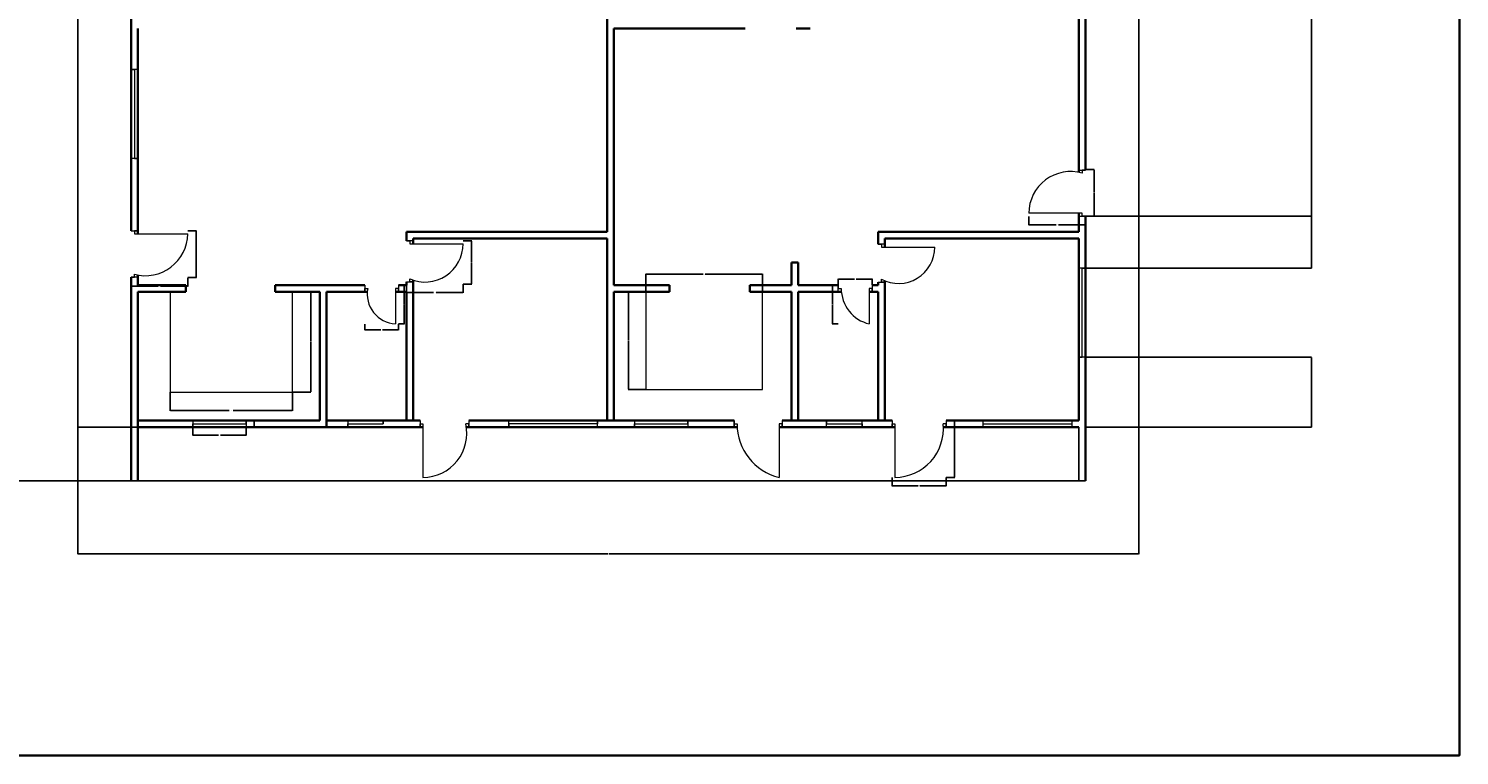
# Model space of a CAD drawing. Units: inches. Extents: x 1520 to 3401, y 1570 to 3432.
# Tile 10 of 15: x 2435 to 3401, y 1570 to 2061. Entities that reach past the tile are written whole.
import ezdxf

# ---------------------------------------------------------------- set-up
doc = ezdxf.new("R2010")
doc.units = ezdxf.units.IN
for name, color, linetype, lineweight in [('A-ANNO-DIMS', 2, 'Continuous', 18), ('A-ANNO-TTLB', 7, 'Continuous', 35), ('A-DOOR', 3, 'Continuous', 18), ('A-FLOR-CASE', 8, 'Continuous', 18), ('A-FLOR-EDGE', 7, 'Continuous', 25), ('A-GLAZ', 4, 'Continuous', 18), ('A-WALL', 7, 'Continuous', 35)]:
    doc.layers.add(name, color=color, linetype=linetype, lineweight=lineweight)
doc.styles.get("Standard").update_dxf_attribs({"font": 'arial.ttf'})
doc.dimstyles.get("Standard").update_dxf_attribs({"dimtxt": 0.18, "dimasz": 0.18, "dimexe": 0.18, "dimexo": 0.0625, "dimgap": 0.09, "dimtad": 0, "dimtih": 1, "dimtoh": 1, "dimdec": 4, "dimzin": 0, "dimdsep": 46, "dimtxsty": 'Standard', "dimcen": 0.09, "dimadec": 0, "dimazin": 0, "dimtfac": 1, "dimtdec": 4, "dimtofl": 0, "dimtmove": 0, "dimatfit": 3, "dimfxl": 1, "dimtolj": 1, "dimtzin": 0, "dimarcsym": 0})

# ---------------------------------------------------------------- blocks, each defined once
blk = doc.blocks.new('DOOR-SWING-24-10')
for p, q in [((0, 21.75), (0, 26.25)), ((0, 26.25), (0, 24)), ((0, 24), (2, 24)), ((23.01, 24), (21.01, 24)), ((21.01, 24), (21.01, 0)), ((23.01, 26.25), (23.01, 21.75)), ((23.01, 21.75), (23.01, 24))]:
    blk.add_line(p, q)
blk.add_arc((26.65, 24), 24.65, 180, 256.77726)
blk = doc.blocks.new('DOOR-SWING-36-11')
for p, q in [((4.5, 26.53), (0, 26.53)), ((0, 26.53), (2.25, 26.53)), ((2.25, 26.53), (2.25, 24.53)), ((2.25, 24.53), (38.25, 24.53)), ((0, 0.83), (4.5, 0.83)), ((2.25, 0.83), (2.25, 2.83)), ((4.5, 0.83), (2.25, 0.83))]:
    blk.add_line(p, q)
blk.add_arc((13.71, 24.53), 24.54, 242.16732, 0)
blk = doc.blocks.new('DOOR-SWING-24-12')
for p, q in [((0, 26.25), (0, 21.75)), ((0, 21.75), (0, 24)), ((0, 24), (2, 24)), ((22.75, 24), (20.75, 24)), ((20.75, 24), (20.75, 0)), ((22.75, 26.25), (22.75, 21.75)), ((22.75, 21.75), (22.75, 24))]:
    blk.add_line(p, q)
blk.add_arc((21.91, 20.23), 20.26, 169.27026, 266.73788)
blk = doc.blocks.new('DOOR-SWING-36-13')
for p, q in [((4.5, 27.75), (0, 27.75)), ((0, 27.75), (2.25, 27.75)), ((2.25, 27.75), (2.25, 25.75)), ((2.25, 25.75), (38.25, 25.75)), ((0, 0.11), (4.5, 0.11)), ((2.25, 0.11), (2.25, 2.11)), ((4.5, 0.11), (2.25, 0.11))]:
    blk.add_line(p, q)
blk.add_arc((12.49, 25.75), 25.76, 246.58617, 0)
blk = doc.blocks.new('DOOR-SWING-36-26')
for p, q in [((0, 31.26), (4.5, 31.26)), ((4.5, 31.26), (2.25, 31.26)), ((2.25, 31.26), (2.25, 29.26)), ((2.25, 29.26), (38.25, 29.26)), ((2.25, 0), (2.25, 2)), ((4.5, 0), (0, 0)), ((0, 0), (2.25, 0))]:
    blk.add_line(p, q)
blk.add_arc((9.61, 29.68), 28.64, 255.11352, 359.16031)
blk = doc.blocks.new('DOOR-SWING-36-27')
for p, q in [((0, 38.25), (0, 33.75)), ((0, 33.75), (0, 36)), ((0, 36), (2, 36)), ((2, 36), (2, 0)), ((36.5, 36), (34.5, 36)), ((36.5, 38.25), (36.5, 33.75)), ((36.5, 33.75), (36.5, 36))]:
    blk.add_line(p, q)
blk.add_arc((2, 32.67), 32.67, 270, 5.84902)
blk = doc.blocks.new('DOOR-SWING-36-28')
for p, q in [((0, 33.75), (0, 38.25)), ((0, 38.25), (0, 33.75)), ((0, 33.75), (0, 36)), ((0, 36), (2, 36)), ((32.37, 36), (30.37, 36)), ((30.37, 36), (30.37, 0)), ((32.37, 38.25), (32.37, 33.75)), ((32.37, 33.75), (32.37, 36))]:
    blk.add_line(p, q)
blk.add_arc((39.03, 36), 37.03, 180, 256.47101)
blk = doc.blocks.new('DOOR-SWING-36-29')
for p, q in [((0, 38.25), (0, 34.72)), ((0, 33.75), (0, 36)), ((0, 36), (2, 36)), ((0, 34.72), (0, 33.75)), ((2, 36), (2, 0)), ((32.89, 36), (30.89, 36)), ((32.89, 38.25), (32.89, 33.75)), ((32.89, 33.75), (32.89, 36))]:
    blk.add_line(p, q)
blk.add_arc((2, 29.59), 29.59, 270, 12.50405)
blk = doc.blocks.new('DOOR-SWING-36-30')
for p, q in [((33.75, 31.05), (38.25, 31.05)), ((38.25, 31.05), (36, 31.05)), ((36, 31.05), (36, 29.05)), ((36, 2), (0, 2)), ((33.75, 0), (38.25, 0)), ((36, 0), (36, 2)), ((38.25, 0), (36, 0))]:
    blk.add_line(p, q)
blk.add_arc((28.16, 2), 28.16, 73.84326, 180)
blk = doc.blocks.new('WIN-PLAN-24-01')
for p, q in [((0, 4.5), (0, 0)), ((0, 0), (0, 2.25)), ((0, 2.25), (24, 2.25)), ((24, 2.25), (24, 4.5)), ((24, 4.5), (24, 0))]:
    blk.add_line(p, q)
blk = doc.blocks.new('WIN-PLAN-60-02')
for p, q in [((4.5, 60), (0, 60)), ((0, 60), (2.25, 60)), ((2.25, 60), (2.25, 0)), ((4.5, 0), (0, 0)), ((2.25, 0), (4.5, 0))]:
    blk.add_line(p, q)
blk = doc.blocks.new('WIN-PLAN-36-04')
for p, q in [((0, 4.5), (0, 0)), ((0, 0), (0, 2.25)), ((0, 2.25), (36, 2.25)), ((36, 2.25), (36, 4.5)), ((36, 4.5), (36, 0))]:
    blk.add_line(p, q)
blk = doc.blocks.new('WIN-PLAN-60-05')
for p, q in [((0, 4.5), (0, 0)), ((0, 2.25), (60, 2.25)), ((60, 4.5), (60, 0))]:
    blk.add_line(p, q)
blk = doc.blocks.new('WIN-PLAN-24-06')
for p, q in [((0, 4.5), (0, 0)), ((0, 0), (0, 2.25)), ((0, 2.25), (24, 2.25)), ((24, 2.25), (24, 4.5)), ((24, 4.5), (24, 2.25))]:
    blk.add_line(p, q)
blk = doc.blocks.new('KITCHEN-COUNTER-01')
for p, q in [((0, 67.75), (0, 0)), ((82.51, 0), (82.51, 67.75)), ((0, 0), (82.51, 0))]:
    blk.add_line(p, q)
blk = doc.blocks.new('KITCHEN-COUNTER-02')
for p, q in [((0, 65.95), (0, 0)), ((78.77, 0), (78.77, 65.95)), ((0, 0), (78.77, 0))]:
    blk.add_line(p, q)
blk = doc.blocks.new('*D71')
at = {"layer": 'A-ANNO-DIMS', "color": 0, "lineweight": -2, "transparency": 16777216}
for p, q in [((2545.58, 1791.62), (2545.58, 1786.1)), ((2581.58, 1791.62), (2581.58, 1786.1)), ((2545.76, 1786.28), (2562.83, 1786.28)), ((2581.4, 1786.28), (2564.34, 1786.28))]:
    blk.add_line(p, q, dxfattribs=at)
at = {"layer": 'A-ANNO-DIMS', "color": 0, "transparency": 16777216}
for points in [[(2545.76, 1786.31), (2545.76, 1786.25), (2545.58, 1786.28)], [(2581.4, 1786.31), (2581.4, 1786.25), (2581.58, 1786.28)]]:
    blk.add_solid(points, dxfattribs=at)
at = {"layer": 'Defpoints', "color": 0, "transparency": 16777216}
for p in [(2545.58, 1791.68), (2581.58, 1791.68), (2581.58, 1786.28)]:
    blk.add_point(p, dxfattribs=at)
at = {"layer": 'A-ANNO-DIMS', "color": 0, "transparency": 16777216, "insert": (2563.58, 1786.28), "char_height": 0.18, "attachment_point": 5}
blk.add_mtext('\\A1;W4 36 TYP.', dxfattribs=at)
blk = doc.blocks.new('*D72')
at = {"layer": 'A-ANNO-DIMS', "color": 0, "lineweight": -2, "transparency": 16777216}
for p, q in [((2581.64, 1796.18), (2587.16, 1796.18)), ((2581.64, 1791.68), (2587.16, 1791.68)), ((2586.98, 1796), (2586.98, 1794.11)), ((2586.98, 1791.86), (2586.98, 1793.75))]:
    blk.add_line(p, q, dxfattribs=at)
at = {"layer": 'A-ANNO-DIMS', "color": 0, "transparency": 16777216}
for points in [[(2586.95, 1796), (2587.01, 1796), (2586.98, 1796.18)], [(2586.95, 1791.86), (2587.01, 1791.86), (2586.98, 1791.68)]]:
    blk.add_solid(points, dxfattribs=at)
at = {"layer": 'Defpoints', "color": 0, "transparency": 16777216}
for p in [(2581.58, 1796.18), (2581.58, 1791.68), (2586.98, 1796.18)]:
    blk.add_point(p, dxfattribs=at)
at = {"layer": 'A-ANNO-DIMS', "color": 0, "transparency": 16777216, "insert": (2586.98, 1793.93), "char_height": 0.18, "attachment_point": 5}
blk.add_mtext('\\A1;5 TYP.', dxfattribs=at)
blk = doc.blocks.new('*D99')
at = {"layer": 'A-ANNO-DIMS', "color": 0, "lineweight": -2, "transparency": 16777216}
for p, q in [((2981.34, 1887.68), (2977.28, 1887.68)), ((2977.46, 1887.5), (2977.46, 1874.74)), ((2977.46, 1861.61), (2977.46, 1874.37)), ((2981.34, 1861.43), (2977.28, 1861.43))]:
    blk.add_line(p, q, dxfattribs=at)
at = {"layer": 'A-ANNO-DIMS', "color": 0, "transparency": 16777216}
for points in [[(2977.43, 1887.5), (2977.49, 1887.5), (2977.46, 1887.68)], [(2977.43, 1861.61), (2977.49, 1861.61), (2977.46, 1861.43)]]:
    blk.add_solid(points, dxfattribs=at)
at = {"layer": 'Defpoints', "color": 0, "transparency": 16777216}
for p in [(2977.46, 1887.68), (2981.4, 1887.68), (2981.4, 1861.43)]:
    blk.add_point(p, dxfattribs=at)
at = {"layer": 'A-ANNO-DIMS', "color": 0, "transparency": 16777216, "insert": (2977.46, 1874.55), "char_height": 0.18, "attachment_point": 5}
blk.add_mtext('\\A1;D10 26 TYP.', dxfattribs=at)
blk = doc.blocks.new('*D100')
at = {"layer": 'A-ANNO-DIMS', "color": 0, "lineweight": -2, "transparency": 16777216}
for p, q in [((2981.4, 1887.74), (2981.4, 1891.8)), ((2981.58, 1891.62), (2992.38, 1891.62)), ((3004.23, 1891.62), (2993.44, 1891.62)), ((3004.41, 1887.74), (3004.41, 1891.8))]:
    blk.add_line(p, q, dxfattribs=at)
at = {"layer": 'A-ANNO-DIMS', "color": 0, "transparency": 16777216}
for points in [[(2981.58, 1891.65), (2981.58, 1891.59), (2981.4, 1891.62)], [(3004.23, 1891.65), (3004.23, 1891.59), (3004.41, 1891.62)]]:
    blk.add_solid(points, dxfattribs=at)
at = {"layer": 'Defpoints', "color": 0, "transparency": 16777216}
for p in [(2981.4, 1887.68), (3004.41, 1891.62), (3004.41, 1887.68)]:
    blk.add_point(p, dxfattribs=at)
at = {"layer": 'A-ANNO-DIMS', "color": 0, "transparency": 16777216, "insert": (2992.91, 1891.62), "char_height": 0.18, "attachment_point": 5}
blk.add_mtext('\\A1;23 TYP.', dxfattribs=at)
blk = doc.blocks.new('*D103')
at = {"layer": 'A-ANNO-DIMS', "color": 0, "lineweight": -2, "transparency": 16777216}
for p, q in [((2684.52, 1887.68), (2688.57, 1887.68)), ((2688.39, 1887.5), (2688.39, 1874.74)), ((2688.39, 1861.61), (2688.39, 1874.37)), ((2684.52, 1861.43), (2688.57, 1861.43))]:
    blk.add_line(p, q, dxfattribs=at)
at = {"layer": 'A-ANNO-DIMS', "color": 0, "transparency": 16777216}
for points in [[(2688.36, 1887.5), (2688.42, 1887.5), (2688.39, 1887.68)], [(2688.36, 1861.61), (2688.42, 1861.61), (2688.39, 1861.43)]]:
    blk.add_solid(points, dxfattribs=at)
at = {"layer": 'Defpoints', "color": 0, "transparency": 16777216}
for p in [(2684.45, 1887.68), (2688.39, 1887.68), (2684.45, 1861.43)]:
    blk.add_point(p, dxfattribs=at)
at = {"layer": 'A-ANNO-DIMS', "color": 0, "transparency": 16777216, "insert": (2688.39, 1874.55), "char_height": 0.18, "attachment_point": 5}
blk.add_mtext('\\A1;D12 26 TYP.', dxfattribs=at)
blk = doc.blocks.new('*D104')
at = {"layer": 'A-ANNO-DIMS', "color": 0, "lineweight": -2, "transparency": 16777216}
for p, q in [((2661.7, 1861.37), (2661.7, 1857.31)), ((2661.88, 1857.49), (2672.55, 1857.49)), ((2684.27, 1857.49), (2673.61, 1857.49)), ((2684.45, 1861.37), (2684.45, 1857.31))]:
    blk.add_line(p, q, dxfattribs=at)
at = {"layer": 'A-ANNO-DIMS', "color": 0, "transparency": 16777216}
for points in [[(2661.88, 1857.52), (2661.88, 1857.46), (2661.7, 1857.49)], [(2684.27, 1857.52), (2684.27, 1857.46), (2684.45, 1857.49)]]:
    blk.add_solid(points, dxfattribs=at)
at = {"layer": 'Defpoints', "color": 0, "transparency": 16777216}
for p in [(2661.7, 1861.43), (2684.45, 1861.43), (2684.45, 1857.49)]:
    blk.add_point(p, dxfattribs=at)
at = {"layer": 'A-ANNO-DIMS', "color": 0, "transparency": 16777216, "insert": (2673.08, 1857.49), "char_height": 0.18, "attachment_point": 5}
blk.add_mtext('\\A1;23 TYP.', dxfattribs=at)
blk = doc.blocks.new('*D105')
at = {"layer": 'A-ANNO-DIMS', "color": 0, "lineweight": -2, "transparency": 16777216}
for p, q in [((2689.9, 1888.32), (2689.9, 1882.46)), ((2728.15, 1888.32), (2728.15, 1882.46)), ((2690.08, 1882.64), (2708.23, 1882.64)), ((2727.97, 1882.64), (2709.81, 1882.64))]:
    blk.add_line(p, q, dxfattribs=at)
at = {"layer": 'A-ANNO-DIMS', "color": 0, "transparency": 16777216}
for points in [[(2690.08, 1882.67), (2690.08, 1882.61), (2689.9, 1882.64)], [(2727.97, 1882.67), (2727.97, 1882.61), (2728.15, 1882.64)]]:
    blk.add_solid(points, dxfattribs=at)
at = {"layer": 'Defpoints', "color": 0, "transparency": 16777216}
for p in [(2689.9, 1888.38), (2728.15, 1888.38), (2728.15, 1882.64)]:
    blk.add_point(p, dxfattribs=at)
at = {"layer": 'A-ANNO-DIMS', "color": 0, "transparency": 16777216, "insert": (2709.02, 1882.64), "char_height": 0.18, "attachment_point": 5}
blk.add_mtext('\\A1;D13 38 TYP.', dxfattribs=at)
blk = doc.blocks.new('*D106')
at = {"layer": 'A-ANNO-DIMS', "color": 0, "lineweight": -2, "transparency": 16777216}
for p, q in [((2728.21, 1917.47), (2734.07, 1917.47)), ((2733.89, 1917.29), (2733.89, 1903.11)), ((2733.89, 1888.56), (2733.89, 1902.74)), ((2728.21, 1888.38), (2734.07, 1888.38))]:
    blk.add_line(p, q, dxfattribs=at)
at = {"layer": 'A-ANNO-DIMS', "color": 0, "transparency": 16777216}
for points in [[(2733.86, 1917.29), (2733.92, 1917.29), (2733.89, 1917.47)], [(2733.86, 1888.56), (2733.92, 1888.56), (2733.89, 1888.38)]]:
    blk.add_solid(points, dxfattribs=at)
at = {"layer": 'Defpoints', "color": 0, "transparency": 16777216}
for p in [(2728.15, 1917.47), (2733.89, 1917.47), (2728.15, 1888.38)]:
    blk.add_point(p, dxfattribs=at)
at = {"layer": 'A-ANNO-DIMS', "color": 0, "transparency": 16777216, "insert": (2733.89, 1902.93), "char_height": 0.18, "attachment_point": 5}
blk.add_mtext('\\A1;29 TYP.', dxfattribs=at)
blk = doc.blocks.new('*D131')
at = {"layer": 'A-ANNO-DIMS', "color": 0, "lineweight": -2, "transparency": 16777216}
for p, q in [((2503.9, 1892.6), (2503.9, 1886.75)), ((2504.08, 1886.93), (2522.23, 1886.93)), ((2541.97, 1886.93), (2523.81, 1886.93)), ((2542.15, 1892.6), (2542.15, 1886.75))]:
    blk.add_line(p, q, dxfattribs=at)
at = {"layer": 'A-ANNO-DIMS', "color": 0, "transparency": 16777216}
for points in [[(2504.08, 1886.96), (2504.08, 1886.9), (2503.9, 1886.93)], [(2541.97, 1886.96), (2541.97, 1886.9), (2542.15, 1886.93)]]:
    blk.add_solid(points, dxfattribs=at)
at = {"layer": 'Defpoints', "color": 0, "transparency": 16777216}
for p in [(2503.9, 1892.67), (2542.15, 1892.67), (2542.15, 1886.93)]:
    blk.add_point(p, dxfattribs=at)
at = {"layer": 'A-ANNO-DIMS', "color": 0, "transparency": 16777216, "insert": (2523.02, 1886.93), "char_height": 0.18, "attachment_point": 5}
blk.add_mtext('\\A1;D26 38 TYP.', dxfattribs=at)
blk = doc.blocks.new('*D132')
at = {"layer": 'A-ANNO-DIMS', "color": 0, "lineweight": -2, "transparency": 16777216}
for p, q in [((2542.21, 1924.2), (2548.07, 1924.2)), ((2547.89, 1924.02), (2547.89, 1908.61)), ((2547.89, 1892.85), (2547.89, 1908.25)), ((2542.21, 1892.67), (2548.07, 1892.67))]:
    blk.add_line(p, q, dxfattribs=at)
at = {"layer": 'A-ANNO-DIMS', "color": 0, "transparency": 16777216}
for points in [[(2547.86, 1924.02), (2547.92, 1924.02), (2547.89, 1924.2)], [(2547.86, 1892.85), (2547.92, 1892.85), (2547.89, 1892.67)]]:
    blk.add_solid(points, dxfattribs=at)
at = {"layer": 'Defpoints', "color": 0, "transparency": 16777216}
for p in [(2542.15, 1924.2), (2547.89, 1924.2), (2542.15, 1892.67)]:
    blk.add_point(p, dxfattribs=at)
at = {"layer": 'A-ANNO-DIMS', "color": 0, "transparency": 16777216, "insert": (2547.89, 1908.43), "char_height": 0.18, "attachment_point": 5}
blk.add_mtext('\\A1;32 TYP.', dxfattribs=at)
blk = doc.blocks.new('*D133')
at = {"layer": 'A-ANNO-DIMS', "color": 0, "lineweight": -2, "transparency": 16777216}
for p, q in [((3054.3, 1796.18), (3060.16, 1796.18)), ((3059.98, 1796), (3059.98, 1777.24)), ((3059.98, 1758.11), (3059.98, 1776.87)), ((3054.3, 1757.93), (3060.16, 1757.93))]:
    blk.add_line(p, q, dxfattribs=at)
at = {"layer": 'A-ANNO-DIMS', "color": 0, "transparency": 16777216}
for points in [[(3059.95, 1796), (3060.01, 1796), (3059.98, 1796.18)], [(3059.95, 1758.11), (3060.01, 1758.11), (3059.98, 1757.93)]]:
    blk.add_solid(points, dxfattribs=at)
at = {"layer": 'Defpoints', "color": 0, "transparency": 16777216}
for p in [(3054.24, 1796.18), (3059.98, 1796.18), (3054.24, 1757.93)]:
    blk.add_point(p, dxfattribs=at)
at = {"layer": 'A-ANNO-DIMS', "color": 0, "transparency": 16777216, "insert": (3059.98, 1777.05), "char_height": 0.18, "attachment_point": 5}
blk.add_mtext('\\A1;D27 38 TYP.', dxfattribs=at)
blk = doc.blocks.new('*D134')
at = {"layer": 'A-ANNO-DIMS', "color": 0, "lineweight": -2, "transparency": 16777216}
for p, q in [((3017.74, 1757.87), (3017.74, 1752.01)), ((3017.92, 1752.19), (3035.46, 1752.19)), ((3054.06, 1752.19), (3036.52, 1752.19)), ((3054.24, 1757.87), (3054.24, 1752.01))]:
    blk.add_line(p, q, dxfattribs=at)
at = {"layer": 'A-ANNO-DIMS', "color": 0, "transparency": 16777216}
for points in [[(3017.92, 1752.22), (3017.92, 1752.16), (3017.74, 1752.19)], [(3054.06, 1752.22), (3054.06, 1752.16), (3054.24, 1752.19)]]:
    blk.add_solid(points, dxfattribs=at)
at = {"layer": 'Defpoints', "color": 0, "transparency": 16777216}
for p in [(3017.74, 1757.93), (3054.24, 1757.93), (3054.24, 1752.19)]:
    blk.add_point(p, dxfattribs=at)
at = {"layer": 'A-ANNO-DIMS', "color": 0, "transparency": 16777216, "insert": (3035.99, 1752.19), "char_height": 0.18, "attachment_point": 5}
blk.add_mtext('\\A1;37 TYP.', dxfattribs=at)
blk = doc.blocks.new('*D139')
at = {"layer": 'A-ANNO-DIMS', "color": 0, "lineweight": -2, "transparency": 16777216}
for p, q in [((3110.15, 1934.02), (3110.15, 1928.17)), ((3148.4, 1934.02), (3148.4, 1928.17)), ((3110.33, 1928.35), (3128.48, 1928.35)), ((3148.22, 1928.35), (3130.06, 1928.35))]:
    blk.add_line(p, q, dxfattribs=at)
at = {"layer": 'A-ANNO-DIMS', "color": 0, "transparency": 16777216}
for points in [[(3110.33, 1928.38), (3110.33, 1928.32), (3110.15, 1928.35)], [(3148.22, 1928.38), (3148.22, 1928.32), (3148.4, 1928.35)]]:
    blk.add_solid(points, dxfattribs=at)
at = {"layer": 'Defpoints', "color": 0, "transparency": 16777216}
for p in [(3110.15, 1934.08), (3148.4, 1934.08), (3148.4, 1928.35)]:
    blk.add_point(p, dxfattribs=at)
at = {"layer": 'A-ANNO-DIMS', "color": 0, "transparency": 16777216, "insert": (3129.27, 1928.35), "char_height": 0.18, "attachment_point": 5}
blk.add_mtext('\\A1;D30 38 TYP.', dxfattribs=at)
blk = doc.blocks.new('*D140')
at = {"layer": 'A-ANNO-DIMS', "color": 0, "lineweight": -2, "transparency": 16777216}
for p, q in [((3148.46, 1965.6), (3154.32, 1965.6)), ((3154.14, 1965.42), (3154.14, 1950.02)), ((3154.14, 1934.26), (3154.14, 1949.66)), ((3148.46, 1934.08), (3154.32, 1934.08))]:
    blk.add_line(p, q, dxfattribs=at)
at = {"layer": 'A-ANNO-DIMS', "color": 0, "transparency": 16777216}
for points in [[(3154.11, 1965.42), (3154.17, 1965.42), (3154.14, 1965.6)], [(3154.11, 1934.26), (3154.17, 1934.26), (3154.14, 1934.08)]]:
    blk.add_solid(points, dxfattribs=at)
at = {"layer": 'Defpoints', "color": 0, "transparency": 16777216}
for p in [(3148.4, 1965.6), (3154.14, 1965.6), (3148.4, 1934.08)]:
    blk.add_point(p, dxfattribs=at)
at = {"layer": 'A-ANNO-DIMS', "color": 0, "transparency": 16777216, "insert": (3154.14, 1949.84), "char_height": 0.18, "attachment_point": 5}
blk.add_mtext('\\A1;32 TYP.', dxfattribs=at)
blk = doc.blocks.new('*D149')
at = {"layer": 'A-ANNO-DIMS', "color": 0, "lineweight": -2, "transparency": 16777216}
for p, q in [((2530.29, 1815.37), (2530.29, 1802.87)), ((2612.81, 1815.37), (2612.81, 1802.87)), ((2530.47, 1803.05), (2570.17, 1803.05)), ((2612.63, 1803.05), (2572.93, 1803.05))]:
    blk.add_line(p, q, dxfattribs=at)
at = {"layer": 'A-ANNO-DIMS', "color": 0, "transparency": 16777216}
for points in [[(2530.47, 1803.08), (2530.47, 1803.02), (2530.29, 1803.05)], [(2612.63, 1803.08), (2612.63, 1803.02), (2612.81, 1803.05)]]:
    blk.add_solid(points, dxfattribs=at)
at = {"layer": 'Defpoints', "color": 0, "transparency": 16777216}
for p in [(2530.29, 1815.43), (2612.81, 1815.43), (2612.81, 1803.05)]:
    blk.add_point(p, dxfattribs=at)
at = {"layer": 'A-ANNO-DIMS', "color": 0, "transparency": 16777216, "insert": (2571.55, 1803.05), "char_height": 0.18, "attachment_point": 5}
blk.add_mtext('\\A1;COUNTER C1 83 TYP.', dxfattribs=at)
blk = doc.blocks.new('*D150')
at = {"layer": 'A-ANNO-DIMS', "color": 0, "lineweight": -2, "transparency": 16777216}
for p, q in [((2612.87, 1883.18), (2625.36, 1883.18)), ((2625.18, 1883), (2625.18, 1849.49)), ((2625.18, 1815.61), (2625.18, 1849.12)), ((2612.87, 1815.43), (2625.36, 1815.43))]:
    blk.add_line(p, q, dxfattribs=at)
at = {"layer": 'A-ANNO-DIMS', "color": 0, "transparency": 16777216}
for points in [[(2625.15, 1883), (2625.21, 1883), (2625.18, 1883.18)], [(2625.15, 1815.61), (2625.21, 1815.61), (2625.18, 1815.43)]]:
    blk.add_solid(points, dxfattribs=at)
at = {"layer": 'Defpoints', "color": 0, "transparency": 16777216}
for p in [(2612.81, 1883.18), (2625.18, 1883.18), (2612.81, 1815.43)]:
    blk.add_point(p, dxfattribs=at)
at = {"layer": 'A-ANNO-DIMS', "color": 0, "transparency": 16777216, "insert": (2625.18, 1849.31), "char_height": 0.18, "attachment_point": 5}
blk.add_mtext('\\A1;68 TYP.', dxfattribs=at)
blk = doc.blocks.new('*D151')
at = {"layer": 'A-ANNO-DIMS', "color": 0, "lineweight": -2, "transparency": 16777216}
for p, q in [((2851.55, 1883.24), (2851.55, 1895.17)), ((2851.73, 1894.99), (2890.22, 1894.99)), ((2930.14, 1894.99), (2891.66, 1894.99)), ((2930.32, 1883.24), (2930.32, 1895.17))]:
    blk.add_line(p, q, dxfattribs=at)
at = {"layer": 'A-ANNO-DIMS', "color": 0, "transparency": 16777216}
for points in [[(2851.73, 1895.02), (2851.73, 1894.96), (2851.55, 1894.99)], [(2930.14, 1895.02), (2930.14, 1894.96), (2930.32, 1894.99)]]:
    blk.add_solid(points, dxfattribs=at)
at = {"layer": 'Defpoints', "color": 0, "transparency": 16777216}
for p in [(2930.32, 1894.99), (2851.55, 1883.18), (2930.32, 1883.18)]:
    blk.add_point(p, dxfattribs=at)
at = {"layer": 'A-ANNO-DIMS', "color": 0, "transparency": 16777216, "insert": (2890.94, 1894.99), "char_height": 0.18, "attachment_point": 5}
blk.add_mtext('\\A1;C2 79 TYP.', dxfattribs=at)
blk = doc.blocks.new('*D152')
at = {"layer": 'A-ANNO-DIMS', "color": 0, "lineweight": -2, "transparency": 16777216}
for p, q in [((2851.49, 1883.18), (2839.56, 1883.18)), ((2839.74, 1883), (2839.74, 1850.38)), ((2839.74, 1817.41), (2839.74, 1850.02)), ((2851.49, 1817.23), (2839.56, 1817.23))]:
    blk.add_line(p, q, dxfattribs=at)
at = {"layer": 'A-ANNO-DIMS', "color": 0, "transparency": 16777216}
for points in [[(2839.71, 1883), (2839.77, 1883), (2839.74, 1883.18)], [(2839.71, 1817.41), (2839.77, 1817.41), (2839.74, 1817.23)]]:
    blk.add_solid(points, dxfattribs=at)
at = {"layer": 'Defpoints', "color": 0, "transparency": 16777216}
for p in [(2839.74, 1883.18), (2851.55, 1883.18), (2851.55, 1817.23)]:
    blk.add_point(p, dxfattribs=at)
at = {"layer": 'A-ANNO-DIMS', "color": 0, "transparency": 16777216, "insert": (2839.74, 1850.2), "char_height": 0.18, "attachment_point": 5}
blk.add_mtext('\\A1;66 TYP.', dxfattribs=at)
blk = doc.blocks.new('*D192')
at = {"layer": 'A-ANNO-DIMS', "color": 0, "lineweight": -2, "transparency": 16777216}
for p, q in [((2467.84, 2733.18), (2386.32, 2733.18)), ((2386.5, 2733), (2386.5, 2244.61)), ((2386.5, 1755.86), (2386.5, 2244.25)), ((2503.84, 1755.68), (2386.32, 1755.68))]:
    blk.add_line(p, q, dxfattribs=at)
at = {"layer": 'A-ANNO-DIMS', "color": 0, "transparency": 16777216}
for points in [[(2386.47, 2733), (2386.53, 2733), (2386.5, 2733.18)], [(2386.47, 1755.86), (2386.53, 1755.86), (2386.5, 1755.68)]]:
    blk.add_solid(points, dxfattribs=at)
at = {"layer": 'Defpoints', "color": 0, "transparency": 16777216}
for p in [(2467.9, 2733.18), (2386.5, 1755.68), (2503.9, 1755.68)]:
    blk.add_point(p, dxfattribs=at)
at = {"layer": 'A-ANNO-DIMS', "color": 0, "transparency": 16777216, "insert": (2386.5, 2244.43), "char_height": 0.18, "attachment_point": 5}
blk.add_mtext('\\A1;977.5', dxfattribs=at)
blk = doc.blocks.new('*D193')
at = {"layer": 'A-ANNO-DIMS', "color": 0, "lineweight": -2, "transparency": 16777216}
for p, q in [((2467.9, 1791.62), (2467.9, 1706.1)), ((3184.4, 1791.62), (3184.4, 1706.1)), ((2468.08, 1706.28), (2825.76, 1706.28)), ((3184.22, 1706.28), (2826.54, 1706.28))]:
    blk.add_line(p, q, dxfattribs=at)
at = {"layer": 'A-ANNO-DIMS', "color": 0, "transparency": 16777216}
for points in [[(2468.08, 1706.31), (2468.08, 1706.25), (2467.9, 1706.28)], [(3184.22, 1706.31), (3184.22, 1706.25), (3184.4, 1706.28)]]:
    blk.add_solid(points, dxfattribs=at)
at = {"layer": 'Defpoints', "color": 0, "transparency": 16777216}
for p in [(2467.9, 1791.68), (3184.4, 1791.68), (3184.4, 1706.28)]:
    blk.add_point(p, dxfattribs=at)
at = {"layer": 'A-ANNO-DIMS', "color": 0, "transparency": 16777216, "insert": (2826.15, 1706.28), "char_height": 0.18, "attachment_point": 5}
blk.add_mtext('\\A1;716.5', dxfattribs=at)
blk = doc.blocks.new('*D194')
at = {"layer": 'A-ANNO-DIMS', "color": 0, "lineweight": -2, "transparency": 16777216}
for p, q in [((3148.46, 1838.98), (3301.09, 1838.98)), ((3300.91, 1838.8), (3300.91, 1815.51)), ((3300.91, 1791.86), (3300.91, 1815.15)), ((3148.46, 1791.68), (3301.09, 1791.68))]:
    blk.add_line(p, q, dxfattribs=at)
at = {"layer": 'A-ANNO-DIMS', "color": 0, "transparency": 16777216}
for points in [[(3300.88, 1838.8), (3300.94, 1838.8), (3300.91, 1838.98)], [(3300.88, 1791.86), (3300.94, 1791.86), (3300.91, 1791.68)]]:
    blk.add_solid(points, dxfattribs=at)
at = {"layer": 'Defpoints', "color": 0, "transparency": 16777216}
for p in [(3148.4, 1838.98), (3300.91, 1838.98), (3148.4, 1791.68)]:
    blk.add_point(p, dxfattribs=at)
at = {"layer": 'A-ANNO-DIMS', "color": 0, "transparency": 16777216, "insert": (3300.91, 1815.33), "char_height": 0.18, "attachment_point": 5}
blk.add_mtext('\\A1;47.3', dxfattribs=at)
blk = doc.blocks.new('*D195')
at = {"layer": 'A-ANNO-DIMS', "color": 0, "lineweight": -2, "transparency": 16777216}
for p, q in [((3148.46, 1934.08), (3301.09, 1934.08)), ((3300.91, 1933.9), (3300.91, 1916.71)), ((3300.91, 1899.16), (3300.91, 1916.35)), ((3148.46, 1898.98), (3301.09, 1898.98))]:
    blk.add_line(p, q, dxfattribs=at)
at = {"layer": 'A-ANNO-DIMS', "color": 0, "transparency": 16777216}
for points in [[(3300.88, 1933.9), (3300.94, 1933.9), (3300.91, 1934.08)], [(3300.88, 1899.16), (3300.94, 1899.16), (3300.91, 1898.98)]]:
    blk.add_solid(points, dxfattribs=at)
at = {"layer": 'Defpoints', "color": 0, "transparency": 16777216}
for p in [(3148.4, 1934.08), (3300.91, 1934.08), (3148.4, 1898.98)]:
    blk.add_point(p, dxfattribs=at)
at = {"layer": 'A-ANNO-DIMS', "color": 0, "transparency": 16777216, "insert": (3300.91, 1916.53), "char_height": 0.18, "attachment_point": 5}
blk.add_mtext('\\A1;35.106', dxfattribs=at)
blk = doc.blocks.new('*D196')
at = {"layer": 'A-ANNO-DIMS', "color": 0, "lineweight": -2, "transparency": 16777216}
for p, q in [((3143.96, 2238.68), (3301.09, 2238.68)), ((3300.91, 2238.5), (3300.91, 2086.56)), ((3300.91, 1934.26), (3300.91, 2086.2)), ((3148.46, 1934.08), (3301.09, 1934.08))]:
    blk.add_line(p, q, dxfattribs=at)
at = {"layer": 'A-ANNO-DIMS', "color": 0, "transparency": 16777216}
for points in [[(3300.88, 2238.5), (3300.94, 2238.5), (3300.91, 2238.68)], [(3300.88, 1934.26), (3300.94, 1934.26), (3300.91, 1934.08)]]:
    blk.add_solid(points, dxfattribs=at)
at = {"layer": 'Defpoints', "color": 0, "transparency": 16777216}
for p in [(3143.9, 2238.68), (3300.91, 2238.68), (3148.4, 1934.08)]:
    blk.add_point(p, dxfattribs=at)
at = {"layer": 'A-ANNO-DIMS', "color": 0, "transparency": 16777216, "insert": (3300.91, 2086.38), "char_height": 0.18, "attachment_point": 5}
blk.add_mtext('\\A1;304.6', dxfattribs=at)

msp = doc.modelspace()

# ---------------------------------------------------------------- linework, layer by layer
at = {"layer": 'A-ANNO-TTLB'}
msp.add_lwpolyline([(1519.9253, 3431.7421), (3400.8761, 3431.7421), (3400.8761, 1570.3458), (1519.9253, 1570.3458)], close=True, dxfattribs=at)
at = {"layer": 'A-FLOR-EDGE'}
for p, q in [((2467.8987, 2733.1786), (2467.8987, 1791.6786)), ((3184.3987, 2733.1786), (3184.3987, 1791.6786)), ((2508.3987, 1791.6786), (2467.8987, 1791.6786)), ((2508.3987, 1791.6786), (2508.3987, 1755.6786)), ((3143.8987, 1791.6786), (3143.8987, 1755.6786)), ((3148.3987, 1791.6786), (3184.3987, 1791.6786)), ((2503.8987, 1755.6786), (3143.8987, 1755.6786)), ((3143.8987, 1755.6786), (3148.3987, 1755.6786))]:
    msp.add_line(p, q, dxfattribs=at)
at = {"layer": 'A-WALL'}
for p, q in [((3143.8987, 2431.1873), (3143.8987, 1963.6868)), ((3148.3987, 2432.7197), (3148.3987, 1965.1342)), ((2825.3987, 1923.6786), (2825.3987, 2234.1786)), ((2503.8987, 2075.1195), (2503.8987, 1924.1968)), ((2503.8987, 2075.1195), (2503.8987, 1924.1968)), ((2508.3987, 2060.6786), (2508.3987, 1922.1968)), ((2918.524, 2060.6786), (2829.8987, 2060.6786)), ((2829.8987, 2060.6786), (2829.8987, 1887.6786)), ((2829.8987, 2060.6786), (2918.524, 2060.6786)), ((2962.3987, 2060.6786), (2953.1027, 2060.6786)), ((2953.1027, 2060.6786), (2957.8987, 2060.6786)), ((2825.3987, 1923.6786), (2825.3987, 2052.6786)), ((3143.8987, 1936.0834), (3143.8987, 1923.6786)), ((3148.3987, 1934.0834), (3148.3987, 1755.6786)), ((2689.8987, 1919.1786), (2689.8987, 1923.6786)), ((2689.8987, 1923.6786), (2825.3987, 1923.6786)), ((3008.3987, 1923.6786), (3143.8987, 1923.6786)), ((3008.3987, 1915.2759), (3008.3987, 1923.6786)), ((2689.8987, 1917.4716), (2689.8987, 1919.1786)), ((2825.3987, 1919.1786), (2694.3987, 1919.1786)), ((2694.3987, 1919.1786), (2694.3987, 1915.4716)), ((2825.3987, 1796.1786), (2825.3987, 1919.1786)), ((3143.8987, 1919.1786), (3012.8987, 1919.1786)), ((3012.8987, 1919.1786), (3012.8987, 1913.2759)), ((3143.8987, 1919.1786), (3143.8987, 1796.1786)), ((2508.3987, 1894.4316), (2508.3987, 1887.6786)), ((2954.3987, 1902.917), (2949.8987, 1902.917)), ((2949.8987, 1902.917), (2949.8987, 1887.6786)), ((2954.3987, 1887.6786), (2954.3987, 1902.917)), ((2503.8987, 1892.9337), (2503.8987, 1755.6786)), ((2503.8987, 1892.9337), (2503.8987, 1755.6786)), ((2540.96, 1887.6786), (2508.3987, 1887.6786)), ((2540.96, 1883.1786), (2540.96, 1887.6786)), ((2661.7006, 1887.6786), (2601.2346, 1887.6786)), ((2601.2346, 1883.1786), (2601.2346, 1887.6786)), ((2689.8987, 1887.6786), (2684.4542, 1887.6786)), ((2689.8987, 1887.6786), (2689.8987, 1889.8302)), ((2694.3987, 1890.9783), (2694.3987, 1887.6786)), ((2694.3987, 1887.6786), (2694.3987, 1796.1786)), ((2867.5204, 1887.6786), (2829.8987, 1887.6786)), ((2867.5204, 1887.6786), (2867.5204, 1883.1786)), ((2949.8987, 1887.6786), (2921.7787, 1887.6786)), ((2921.7787, 1887.6786), (2921.7787, 1883.1786)), ((2981.3987, 1887.6786), (2954.3987, 1887.6786)), ((3008.3987, 1887.6786), (3004.4131, 1887.6786)), ((3008.3987, 1887.6786), (3008.3987, 1889.5733)), ((3012.8987, 1890.5272), (3012.8987, 1887.6786)), ((3012.8987, 1887.6786), (3012.8987, 1796.1786)), ((2508.3987, 1883.1786), (2508.3987, 1755.6786)), ((2540.96, 1883.1786), (2508.3987, 1883.1786)), ((2631.3987, 1883.1786), (2601.2346, 1883.1786)), ((2631.3987, 1883.1786), (2631.3987, 1796.1786)), ((2635.8987, 1883.1786), (2635.8987, 1791.6786)), ((2663.4036, 1883.1786), (2635.8987, 1883.1786)), ((2689.8987, 1883.1786), (2682.4542, 1883.1786)), ((2689.8987, 1796.1786), (2689.8987, 1883.1786)), ((2867.5204, 1883.1786), (2829.8987, 1883.1786)), ((2829.8987, 1883.1786), (2829.8987, 1796.1786)), ((2829.8987, 1883.1786), (2867.5204, 1883.1786)), ((2949.8987, 1883.1786), (2921.7787, 1883.1786)), ((2921.7787, 1883.1786), (2949.8987, 1883.1786)), ((2949.8987, 1883.1786), (2949.8987, 1796.1786)), ((2983.5015, 1883.1786), (2954.3987, 1883.1786)), ((2954.3987, 1796.1786), (2954.3987, 1883.1786)), ((3008.3987, 1883.1786), (3002.4131, 1883.1786)), ((3008.3987, 1796.1786), (3008.3987, 1883.1786)), ((2631.3987, 1796.1786), (2508.3987, 1796.1786)), ((2701.0136, 1791.6786), (2508.3987, 1791.6786)), ((2699.0136, 1796.1786), (2635.8987, 1796.1786)), ((2635.8987, 1796.1786), (2689.8987, 1796.1786)), ((2694.3987, 1796.1786), (2699.0136, 1796.1786)), ((2913.1626, 1791.6786), (2730.3117, 1791.6786)), ((2911.0942, 1796.1786), (2731.9032, 1796.1786)), ((2731.9032, 1796.1786), (2825.3987, 1796.1786)), ((3019.7397, 1791.6786), (2941.4595, 1791.6786)), ((3017.7397, 1796.1786), (2943.4595, 1796.1786)), ((2949.8987, 1796.1786), (2954.3987, 1796.1786)), ((2954.3987, 1796.1786), (3008.3987, 1796.1786)), ((3143.8987, 1791.6786), (3052.3924, 1791.6786)), ((3143.8987, 1796.1786), (3054.2402, 1796.1786))]:
    msp.add_line(p, q, dxfattribs=at)

# ---------------------------------------------------------------- block references
at = {"layer": 'A-DOOR'}
for name, p in [('DOOR-SWING-36-30', (3110.1488, 1934.083)), ('DOOR-SWING-36-26', (2503.8988, 1892.934)), ('DOOR-SWING-36-13', (2689.8988, 1889.717)), ('DOOR-SWING-36-11', (3008.3988, 1888.744)), ('DOOR-SWING-24-12', (2661.7008, 1861.429)), ('DOOR-SWING-24-10', (2981.3988, 1861.429)), ('DOOR-SWING-36-29', (2699.0138, 1757.93)), ('DOOR-SWING-36-28', (2911.0938, 1757.929)), ('DOOR-SWING-36-27', (3017.7398, 1757.929))]:
    msp.add_blockref(name, p, dxfattribs=at)
at = {"layer": 'A-FLOR-CASE'}
for name, p in [('KITCHEN-COUNTER-01', (2530.2918, 1815.432)), ('KITCHEN-COUNTER-02', (2851.5548, 1817.227))]:
    msp.add_blockref(name, p, dxfattribs=at)
at = {"layer": 'A-GLAZ'}
for name, p in [('WIN-PLAN-60-02', (2503.8988, 1973.002)), ('WIN-PLAN-36-04', (2545.5823, 1791.679)), ('WIN-PLAN-24-06', (2650.2408, 1791.679)), ('WIN-PLAN-36-04', (2843.7798, 1791.679)), ('WIN-PLAN-60-05', (3079.1708, 1791.679))]:
    msp.add_blockref(name, p, dxfattribs=at)
at = {"layer": 'A-GLAZ', "extrusion": (0, 0, -1), "zscale": -1, "rotation": 180}
for name, p in [('WIN-PLAN-60-02', (-3143.8988, 1898.9765)), ('WIN-PLAN-24-01', (-2973.5133, 1796.1783))]:
    msp.add_blockref(name, p, dxfattribs=at)
at = {"layer": 'A-GLAZ', "rotation": 270}
msp.add_blockref('WIN-PLAN-60-02', (2758.9281, 1796.1785), dxfattribs=at)

# ---------------------------------------------------------------- dimensions: what is measured, and where the dimension line sits
at = {"layer": 'A-ANNO-DIMS'}
for base, p1, p2, override, picture, middle in [((2386.4982, 1755.6786), (2467.8987, 2733.1786), (2503.8987, 1755.6786), {"dimdec": 1, "dimlfac": 1, "dimrnd": 0, "dimzin": 0, "dimdsep": 46, "dimlunit": 2}, '*D192', (2386.4982, 2244.4286)), ((3300.9148, 2238.6786), (3148.3987, 1934.0834), (3143.8987, 2238.6786), {"dimdec": 1, "dimlfac": 1, "dimrnd": 0, "dimzin": 0, "dimdsep": 46, "dimlunit": 2}, '*D196', (3300.9148, 2086.381)), ((3300.9148, 1934.0834), (3148.3987, 1898.977), (3148.3987, 1934.0834), {"dimdec": 3, "dimlfac": 1, "dimrnd": 0, "dimzin": 0, "dimdsep": 46, "dimlunit": 2}, '*D195', (3300.9148, 1916.5302)), ((3300.9148, 1838.977), (3148.3987, 1791.6786), (3148.3987, 1838.977), {"dimdec": 1, "dimlfac": 1, "dimrnd": 0, "dimzin": 0, "dimdsep": 46, "dimlunit": 2}, '*D194', (3300.9148, 1815.3278))]:
    dim = msp.add_linear_dim(base=base, p1=p1, p2=p2, angle=90, dimstyle='Standard', override=override, dxfattribs=at)
    dim.commit()
    dim.dimension.update_dxf_attribs({"geometry": picture, "text_midpoint": middle})
for base, p1, p2, text, picture, middle in [((3154.1362, 1965.5984), (3148.3987, 1934.0834), (3148.3987, 1965.5984), '<> TYP.', '*D140', (3154.1362, 1949.8409)), ((2547.8862, 1924.1968), (2542.1487, 1892.6674), (2542.1487, 1924.1968), '<> TYP.', '*D132', (2547.8862, 1908.4321)), ((2733.8862, 1917.4716), (2728.1487, 1888.3822), (2728.1487, 1917.4716), '<> TYP.', '*D106', (2733.8862, 1902.9269)), ((2688.3917, 1887.6786), (2684.4542, 1861.4286), (2684.4542, 1887.6786), 'D12 <> TYP.', '*D103', (2688.3917, 1874.5536)), ((2977.4612, 1887.6786), (2981.3987, 1861.4286), (2981.3987, 1887.6786), 'D10 <> TYP.', '*D99', (2977.4612, 1874.5536)), ((2625.1839, 1883.1786), (2612.8067, 1815.4317), (2612.8067, 1883.1786), '<> TYP.', '*D150', (2625.1839, 1849.3052)), ((2839.7399, 1883.1786), (2851.5548, 1817.2271), (2851.5548, 1883.1786), '<> TYP.', '*D152', (2839.7399, 1850.2029)), ((2586.9824566077, 1796.1786294992), (2581.5824566077, 1791.6786294992), (2581.5824566077, 1796.1786294992), '<> TYP.', '*D72', (2586.9824566077, 1793.9286294992)), ((3059.9777, 1796.1786), (3054.2402, 1757.9286), (3054.2402, 1796.1786), 'D27 <> TYP.', '*D133', (3059.9777, 1777.0536))]:
    dim = msp.add_linear_dim(base=base, p1=p1, p2=p2, angle=90, text=text, dimstyle='Standard', override={"dimdec": 0, "dimlfac": 1, "dimrnd": 0, "dimzin": 0, "dimdsep": 46, "dimlunit": 2}, dxfattribs=at)
    dim.commit()
    dim.dimension.update_dxf_attribs({"geometry": picture, "text_midpoint": middle})
for base, p1, p2, text, picture, middle in [((3148.3987, 1928.3459), (3110.1487, 1934.0834), (3148.3987, 1934.0834), 'D30 <> TYP.', '*D139', (3129.2737, 1928.3459)), ((2930.3207, 1894.9935), (2851.5548, 1883.1786), (2930.3207, 1883.1786), 'C2 <> TYP.', '*D151', (2890.9377, 1894.9935)), ((2542.1487, 1886.9299), (2503.8987, 1892.6674), (2542.1487, 1892.6674), 'D26 <> TYP.', '*D131', (2523.0237, 1886.9299)), ((2728.1487, 1882.6447), (2689.8987, 1888.3822), (2728.1487, 1888.3822), 'D13 <> TYP.', '*D105', (2709.0237, 1882.6447)), ((3004.4131, 1891.6161), (2981.3987, 1887.6786), (3004.4131, 1887.6786), '<> TYP.', '*D100', (2992.9059, 1891.6161)), ((2684.4542, 1857.4911), (2661.7006, 1861.4286), (2684.4542, 1861.4286), '<> TYP.', '*D104', (2673.0774, 1857.4911)), ((2612.8067, 1803.0545), (2530.2921, 1815.4317), (2612.8067, 1815.4317), 'COUNTER C1 <> TYP.', '*D149', (2571.5494, 1803.0545)), ((2581.5825, 1786.2786), (2545.5825, 1791.6786), (2581.5825, 1791.6786), 'W4 <> TYP.', '*D71', (2563.5825, 1786.2786)), ((3054.2402, 1752.1911), (3017.7397, 1757.9286), (3054.2402, 1757.9286), '<> TYP.', '*D134', (3035.9899, 1752.1911))]:
    dim = msp.add_linear_dim(base=base, p1=p1, p2=p2, text=text, dimstyle='Standard', override={"dimdec": 0, "dimlfac": 1, "dimrnd": 0, "dimzin": 0, "dimdsep": 46, "dimlunit": 2}, dxfattribs=at)
    dim.commit()
    dim.dimension.update_dxf_attribs({"geometry": picture, "text_midpoint": middle})
dim = msp.add_linear_dim(base=(3184.3987, 1706.2786), p1=(2467.8987, 1791.6786), p2=(3184.3987, 1791.6786), dimstyle='Standard', override={"dimdec": 1, "dimlfac": 1, "dimrnd": 0, "dimzin": 0, "dimdsep": 46, "dimlunit": 2}, dxfattribs=at)
dim.commit()
dim.dimension.update_dxf_attribs({"geometry": '*D193', "text_midpoint": (2826.1487, 1706.2786)})

doc.saveas('drawing.dxf')
